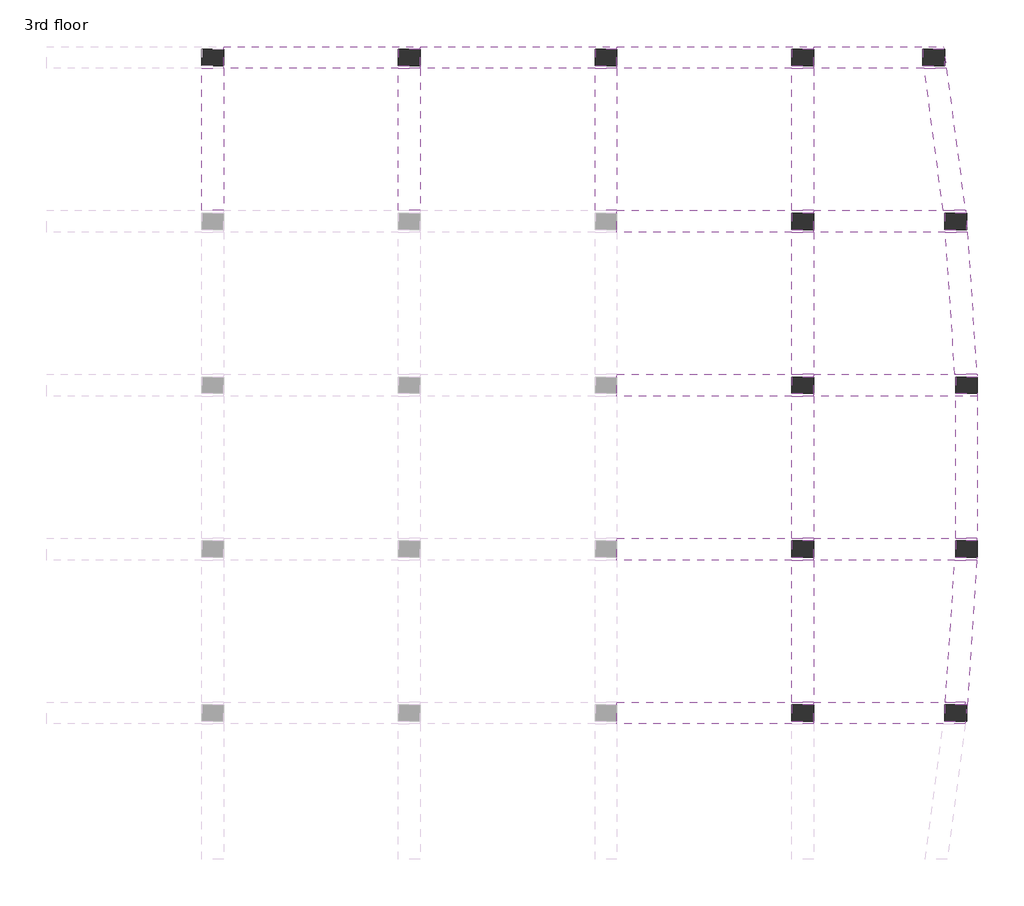
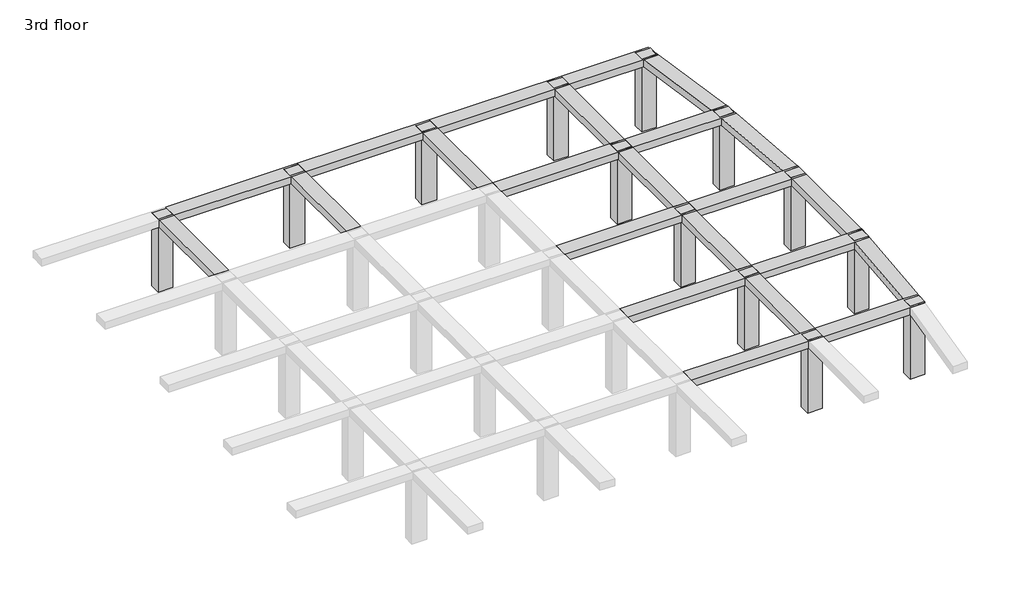
# One storey, part 3 of 3: 23 beams, 13 columns.
"""IFC4 building model written with IfcOpenShell, lengths in millimetres."""

from ifc_helpers import new_model, si_unit, frame, origin, place, context, project, spatial, polyline, outline, extrude, faceted_brep, element, save

model = new_model("IFC4")

# Units and contexts
model_context = context("Model", 3, world=origin())
ifc_project = project(units=[si_unit("LENGTHUNIT", "METRE", prefix="MILLI")], contexts=[model_context])

# Site, building, storey
site = spatial("IfcSite", under=ifc_project)
building = spatial("IfcBuilding", under=site)
storey = spatial("IfcBuildingStorey", under=building, Name="3rd floor", Elevation=9601.2)

# Beams
placement = place(None, origin())
element("IfcBeam", 1, ObjectType="Concrete-Rectangular Beam : 2' x2'", at=placement, inside=storey, context=model_context, shape_type="Brep", body=[
    faceted_brep([(-160.074232, 1680.7831222, 12801.6), (-160.074232, 1604.5831222, 12801.6), (-160.074232, 1147.3831222, 12801.6), (-160.074232, 1071.1831222, 12801.6), (4716.725768, 1071.1831222, 12801.6), (5326.325768, 1071.1831222, 12801.6), (5326.325768, 1147.3831222, 12801.6), (4716.725768, 1147.3831222, 12801.6), (4716.725768, 1604.5831222, 12801.6), (5326.325768, 1604.5831222, 12801.6), (5326.325768, 1680.7831222, 12801.6), (4716.725768, 1680.7831222, 12801.6), (-160.074232, 1071.1831222, 12496.8), (4716.725768, 1071.1831222, 12496.8), (5326.325768, 1071.1831222, 12496.8), (-160.074232, 1147.3831222, 12496.8), (-160.074232, 1604.5831222, 12496.8), (-160.074232, 1680.7831222, 12496.8), (4716.725768, 1680.7831222, 12496.8), (5326.325768, 1680.7831222, 12496.8), (5326.325768, 1604.5831222, 12496.8), (4716.725768, 1604.5831222, 12496.8), (4716.725768, 1147.3831222, 12496.8), (5326.325768, 1147.3831222, 12496.8)], [[[0, 1, 2, 3, 4, 5, 6, 7, 8, 9, 10, 11]], [[3, 12, 13, 14, 5, 4]], [[12, 15, 16, 17, 18, 19, 20, 21, 22, 23, 14, 13]], [[10, 19, 18, 17, 0, 11]], [[3, 2, 1, 0, 17, 16, 15, 12]], [[5, 14, 23, 6]], [[22, 7, 6, 23]], [[7, 22, 21, 8]], [[8, 21, 20, 9]], [[19, 10, 9, 20]]]),
])
element("IfcBeam", 2, ObjectType="Concrete-Rectangular Beam : 2' x2'", at=placement, inside=storey, context=model_context, shape_type="Brep", body=[
    faceted_brep([(9555.2251658, 1680.7831222, 12801.6), (9003.0522312, 1680.7831222, 12801.6), (5326.325768, 1680.7831222, 12801.6), (5326.325768, 1604.5831222, 12801.6), (5326.325768, 1147.3831222, 12801.6), (5326.325768, 1071.1831222, 12801.6), (8940.2370643, 1071.1831222, 12801.6), (9555.2251658, 1071.1831222, 12801.6), (9555.2251658, 1147.3831222, 12801.6), (8983.5457827, 1147.3831222, 12801.6), (8983.5457827, 1604.5831222, 12801.6), (9555.2251658, 1604.5831222, 12801.6), (9555.2251658, 1071.1831222, 12496.8), (5326.325768, 1071.1831222, 12496.8), (8940.2370643, 1071.1831222, 12496.8), (5326.325768, 1147.3831222, 12496.8), (5326.325768, 1604.5831222, 12496.8), (5326.325768, 1680.7831222, 12496.8), (9003.0522312, 1680.7831222, 12496.8), (9555.2251658, 1680.7831222, 12496.8), (9555.2251658, 1604.5831222, 12496.8), (8983.5457827, 1604.5831222, 12496.8), (8983.5457827, 1147.3831222, 12496.8), (9555.2251658, 1147.3831222, 12496.8)], [[[0, 1, 2, 3, 4, 5, 6, 7, 8, 9, 10, 11]], [[12, 7, 6, 5, 13, 14]], [[12, 14, 13, 15, 16, 17, 18, 19, 20, 21, 22, 23]], [[0, 19, 18, 17, 2, 1]], [[7, 12, 23, 8]], [[5, 4, 3, 2, 17, 16, 15, 13]], [[22, 9, 8, 23]], [[9, 22, 21, 10]], [[10, 21, 20, 11]], [[19, 0, 11, 20]]]),
])
element("IfcBeam", 3, ObjectType="Concrete-Rectangular Beam : 2' x2'", at=placement, inside=storey, context=model_context, shape_type="Brep", body=[
    faceted_brep([(-160.074232, 6252.7831222, 12801.6), (-160.074232, 6176.5831222, 12801.6), (-160.074232, 5719.3831222, 12801.6), (-160.074232, 5643.1831222, 12801.6), (4716.725768, 5643.1831222, 12801.6), (5326.325768, 5643.1831222, 12801.6), (5326.325768, 5719.3831222, 12801.6), (4716.725768, 5719.3831222, 12801.6), (4716.725768, 6176.5831222, 12801.6), (5326.325768, 6176.5831222, 12801.6), (5326.325768, 6252.7831222, 12801.6), (4716.725768, 6252.7831222, 12801.6), (-160.074232, 5643.1831222, 12496.8), (4716.725768, 5643.1831222, 12496.8), (5326.325768, 5643.1831222, 12496.8), (-160.074232, 5719.3831222, 12496.8), (-160.074232, 6176.5831222, 12496.8), (-160.074232, 6252.7831222, 12496.8), (4716.725768, 6252.7831222, 12496.8), (5326.325768, 6252.7831222, 12496.8), (5326.325768, 6176.5831222, 12496.8), (4716.725768, 6176.5831222, 12496.8), (4716.725768, 5719.3831222, 12496.8), (5326.325768, 5719.3831222, 12496.8)], [[[0, 1, 2, 3, 4, 5, 6, 7, 8, 9, 10, 11]], [[3, 12, 13, 14, 5, 4]], [[12, 15, 16, 17, 18, 19, 20, 21, 22, 23, 14, 13]], [[10, 19, 18, 17, 0, 11]], [[3, 2, 1, 0, 17, 16, 15, 12]], [[5, 14, 23, 6]], [[22, 7, 6, 23]], [[7, 22, 21, 8]], [[8, 21, 20, 9]], [[19, 10, 9, 20]]]),
])
element("IfcBeam", 4, ObjectType="Concrete-Rectangular Beam : 2' x2'", at=placement, inside=storey, context=model_context, shape_type="Brep", body=[
    faceted_brep([(9876.2389574, 6252.7831222, 12801.6), (9286.1454059, 6252.7831222, 12801.6), (5326.325768, 6252.7831222, 12801.6), (5326.325768, 6176.5831222, 12801.6), (5326.325768, 5719.3831222, 12801.6), (5326.325768, 5643.1831222, 12801.6), (9265.305238, 5643.1831222, 12801.6), (9876.2389574, 5643.1831222, 12801.6), (9876.2389574, 5719.3831222, 12801.6), (9286.1454059, 5719.3831222, 12801.6), (9286.1454059, 6176.5831222, 12801.6), (9876.2389574, 6176.5831222, 12801.6), (9876.2389574, 5643.1831222, 12496.8), (5326.325768, 5643.1831222, 12496.8), (9265.305238, 5643.1831222, 12496.8), (5326.325768, 5719.3831222, 12496.8), (5326.325768, 6176.5831222, 12496.8), (5326.325768, 6252.7831222, 12496.8), (9286.1454059, 6252.7831222, 12496.8), (9876.2389574, 6252.7831222, 12496.8), (9876.2389574, 6176.5831222, 12496.8), (9286.1454059, 6176.5831222, 12496.8), (9286.1454059, 5719.3831222, 12496.8), (9876.2389574, 5719.3831222, 12496.8)], [[[0, 1, 2, 3, 4, 5, 6, 7, 8, 9, 10, 11]], [[12, 7, 6, 5, 13, 14]], [[12, 14, 13, 15, 16, 17, 18, 19, 20, 21, 22, 23]], [[0, 19, 18, 17, 2, 1]], [[7, 12, 23, 8]], [[5, 4, 3, 2, 17, 16, 15, 13]], [[22, 9, 8, 23]], [[9, 22, 21, 10]], [[10, 21, 20, 11]], [[19, 0, 11, 20]]]),
])
element("IfcBeam", 5, ObjectType="Concrete-Rectangular Beam : 2' x2'", at=placement, inside=storey, context=model_context, shape_type="Brep", body=[
    faceted_brep([(-160.074232, 10824.7831222, 12801.6), (-160.074232, 10748.5831222, 12801.6), (-160.074232, 10291.3831222, 12801.6), (-160.074232, 10215.1831222, 12801.6), (4716.725768, 10215.1831222, 12801.6), (5326.325768, 10215.1831222, 12801.6), (5326.325768, 10291.3831222, 12801.6), (4716.725768, 10291.3831222, 12801.6), (4716.725768, 10748.5831222, 12801.6), (5326.325768, 10748.5831222, 12801.6), (5326.325768, 10824.7831222, 12801.6), (4716.725768, 10824.7831222, 12801.6), (-160.074232, 10215.1831222, 12496.8), (4716.725768, 10215.1831222, 12496.8), (5326.325768, 10215.1831222, 12496.8), (-160.074232, 10291.3831222, 12496.8), (-160.074232, 10748.5831222, 12496.8), (-160.074232, 10824.7831222, 12496.8), (4716.725768, 10824.7831222, 12496.8), (5326.325768, 10824.7831222, 12496.8), (5326.325768, 10748.5831222, 12496.8), (4716.725768, 10748.5831222, 12496.8), (4716.725768, 10291.3831222, 12496.8), (5326.325768, 10291.3831222, 12496.8)], [[[0, 1, 2, 3, 4, 5, 6, 7, 8, 9, 10, 11]], [[3, 12, 13, 14, 5, 4]], [[12, 15, 16, 17, 18, 19, 20, 21, 22, 23, 14, 13]], [[10, 19, 18, 17, 0, 11]], [[3, 2, 1, 0, 17, 16, 15, 12]], [[5, 14, 23, 6]], [[22, 7, 6, 23]], [[7, 22, 21, 8]], [[8, 21, 20, 9]], [[19, 10, 9, 20]]]),
])
element("IfcBeam", 6, ObjectType="Concrete-Rectangular Beam : 2' x2'", at=placement, inside=storey, context=model_context, shape_type="Brep", body=[
    faceted_brep([(9895.7454059, 10824.7831222, 12801.6), (9876.2389574, 10824.7831222, 12801.6), (9265.305238, 10824.7831222, 12801.6), (5326.325768, 10824.7831222, 12801.6), (5326.325768, 10748.5831222, 12801.6), (5326.325768, 10291.3831222, 12801.6), (5326.325768, 10215.1831222, 12801.6), (9895.7454059, 10215.1831222, 12801.6), (9895.7454059, 10291.3831222, 12801.6), (9286.1454059, 10291.3831222, 12801.6), (9286.1454059, 10748.5831222, 12801.6), (9895.7454059, 10748.5831222, 12801.6), (9895.7454059, 10215.1831222, 12496.8), (5326.325768, 10215.1831222, 12496.8), (5326.325768, 10291.3831222, 12496.8), (5326.325768, 10748.5831222, 12496.8), (5326.325768, 10824.7831222, 12496.8), (9265.305238, 10824.7831222, 12496.8), (9876.2389574, 10824.7831222, 12496.8), (9895.7454059, 10824.7831222, 12496.8), (9895.7454059, 10748.5831222, 12496.8), (9286.1454059, 10748.5831222, 12496.8), (9286.1454059, 10291.3831222, 12496.8), (9895.7454059, 10291.3831222, 12496.8)], [[[0, 1, 2, 3, 4, 5, 6, 7, 8, 9, 10, 11]], [[12, 7, 6, 13]], [[12, 13, 14, 15, 16, 17, 18, 19, 20, 21, 22, 23]], [[0, 19, 18, 17, 16, 3, 2, 1]], [[7, 12, 23, 8]], [[6, 5, 4, 3, 16, 15, 14, 13]], [[22, 9, 8, 23]], [[9, 22, 21, 10]], [[10, 21, 20, 11]], [[19, 0, 11, 20]]]),
])
element("IfcBeam", 7, ObjectType="Concrete-Rectangular Beam : 2' x2'", at=placement, inside=storey, context=model_context, shape_type="Brep", body=[
    faceted_brep([(-160.074232, 15396.7831222, 12801.6), (-160.074232, 15320.5831222, 12801.6), (-160.074232, 14863.3831222, 12801.6), (-160.074232, 14787.1831222, 12801.6), (4716.725768, 14787.1831222, 12801.6), (5326.325768, 14787.1831222, 12801.6), (5326.325768, 14863.3831222, 12801.6), (4716.725768, 14863.3831222, 12801.6), (4716.725768, 15320.5831222, 12801.6), (5326.325768, 15320.5831222, 12801.6), (5326.325768, 15396.7831222, 12801.6), (4716.725768, 15396.7831222, 12801.6), (-160.074232, 14787.1831222, 12496.8), (4716.725768, 14787.1831222, 12496.8), (5326.325768, 14787.1831222, 12496.8), (-160.074232, 14863.3831222, 12496.8), (-160.074232, 15320.5831222, 12496.8), (-160.074232, 15396.7831222, 12496.8), (4716.725768, 15396.7831222, 12496.8), (5326.325768, 15396.7831222, 12496.8), (5326.325768, 15320.5831222, 12496.8), (4716.725768, 15320.5831222, 12496.8), (4716.725768, 14863.3831222, 12496.8), (5326.325768, 14863.3831222, 12496.8)], [[[0, 1, 2, 3, 4, 5, 6, 7, 8, 9, 10, 11]], [[3, 12, 13, 14, 5, 4]], [[12, 15, 16, 17, 18, 19, 20, 21, 22, 23, 14, 13]], [[10, 19, 18, 17, 0, 11]], [[3, 2, 1, 0, 17, 16, 15, 12]], [[5, 14, 23, 6]], [[22, 7, 6, 23]], [[7, 22, 21, 8]], [[8, 21, 20, 9]], [[19, 10, 9, 20]]]),
])
element("IfcBeam", 8, ObjectType="Concrete-Rectangular Beam : 2' x2'", at=placement, inside=storey, context=model_context, shape_type="Brep", body=[
    faceted_brep([(9573.6393342, 15396.7831222, 12801.6), (9555.2251658, 15396.7831222, 12801.6), (8940.2370643, 15396.7831222, 12801.6), (5326.325768, 15396.7831222, 12801.6), (5326.325768, 15320.5831222, 12801.6), (5326.325768, 14863.3831222, 12801.6), (5326.325768, 14787.1831222, 12801.6), (9003.0522312, 14787.1831222, 12801.6), (9613.9859506, 14787.1831222, 12801.6), (9593.1457827, 15102.0587543, 12801.6), (9593.1457827, 14863.3831222, 12801.6), (8983.5457827, 14863.3831222, 12801.6), (8983.5457827, 15320.5831222, 12801.6), (9578.6826612, 15320.5831222, 12801.6), (9613.9859506, 14787.1831222, 12496.8), (5326.325768, 14787.1831222, 12496.8), (9003.0522312, 14787.1831222, 12496.8), (5326.325768, 14863.3831222, 12496.8), (5326.325768, 15320.5831222, 12496.8), (5326.325768, 15396.7831222, 12496.8), (8940.2370643, 15396.7831222, 12496.8), (9555.2251658, 15396.7831222, 12496.8), (9573.6393342, 15396.7831222, 12496.8), (9578.6826612, 15320.5831222, 12496.8), (8983.5457827, 15320.5831222, 12496.8), (8983.5457827, 14863.3831222, 12496.8), (9593.1457827, 14863.3831222, 12496.8), (9593.1457827, 15102.0587543, 12496.8)], [[[0, 1, 2, 3, 4, 5, 6, 7, 8, 9, 10, 11, 12, 13]], [[14, 8, 7, 6, 15, 16]], [[14, 16, 15, 17, 18, 19, 20, 21, 22, 23, 24, 25, 26, 27]], [[0, 22, 21, 20, 19, 3, 2, 1]], [[8, 14, 27, 9]], [[6, 5, 4, 3, 19, 18, 17, 15]], [[26, 10, 9, 27]], [[10, 26, 25, 11]], [[11, 25, 24, 12]], [[12, 24, 23, 13]], [[22, 0, 13, 23]]]),
])
element("IfcBeam", 9, ObjectType="Concrete-Rectangular Beam : 2' x2'", at=placement, inside=storey, context=model_context, shape_type="Brep", body=[
    faceted_brep([(-11132.874232, 19968.7831222, 12801.6), (-11132.874232, 19892.5831222, 12801.6), (-11132.874232, 19435.3831222, 12801.6), (-11132.874232, 19359.1831222, 12801.6), (-6256.074232, 19359.1831222, 12801.6), (-5646.474232, 19359.1831222, 12801.6), (-5646.474232, 19435.3831222, 12801.6), (-6256.074232, 19435.3831222, 12801.6), (-6256.074232, 19892.5831222, 12801.6), (-5646.474232, 19892.5831222, 12801.6), (-5646.474232, 19968.7831222, 12801.6), (-11132.874232, 19359.1831222, 12496.8), (-6256.074232, 19359.1831222, 12496.8), (-5646.474232, 19359.1831222, 12496.8), (-11132.874232, 19435.3831222, 12496.8), (-11132.874232, 19892.5831222, 12496.8), (-11132.874232, 19968.7831222, 12496.8), (-5646.474232, 19968.7831222, 12496.8), (-5646.474232, 19892.5831222, 12496.8), (-6256.074232, 19892.5831222, 12496.8), (-6256.074232, 19435.3831222, 12496.8), (-5646.474232, 19435.3831222, 12496.8)], [[[0, 1, 2, 3, 4, 5, 6, 7, 8, 9, 10]], [[3, 11, 12, 13, 5, 4]], [[11, 14, 15, 16, 17, 18, 19, 20, 21, 13, 12]], [[10, 17, 16, 0]], [[3, 2, 1, 0, 16, 15, 14, 11]], [[5, 13, 21, 6]], [[20, 7, 6, 21]], [[7, 20, 19, 8]], [[8, 19, 18, 9]], [[17, 10, 9, 18]]]),
])
element("IfcBeam", 10, ObjectType="Concrete-Rectangular Beam : 2' x2'", at=placement, inside=storey, context=model_context, shape_type="Brep", body=[
    faceted_brep([(-160.074232, 19968.7831222, 12801.6), (-5646.474232, 19968.7831222, 12801.6), (-5646.474232, 19892.5831222, 12801.6), (-5646.474232, 19435.3831222, 12801.6), (-5646.474232, 19359.1831222, 12801.6), (-769.674232, 19359.1831222, 12801.6), (-160.074232, 19359.1831222, 12801.6), (-160.074232, 19435.3831222, 12801.6), (-769.674232, 19435.3831222, 12801.6), (-769.674232, 19892.5831222, 12801.6), (-160.074232, 19892.5831222, 12801.6), (-160.074232, 19359.1831222, 12496.8), (-5646.474232, 19359.1831222, 12496.8), (-769.674232, 19359.1831222, 12496.8), (-5646.474232, 19435.3831222, 12496.8), (-5646.474232, 19892.5831222, 12496.8), (-5646.474232, 19968.7831222, 12496.8), (-160.074232, 19968.7831222, 12496.8), (-160.074232, 19892.5831222, 12496.8), (-769.674232, 19892.5831222, 12496.8), (-769.674232, 19435.3831222, 12496.8), (-160.074232, 19435.3831222, 12496.8)], [[[0, 1, 2, 3, 4, 5, 6, 7, 8, 9, 10]], [[11, 6, 5, 4, 12, 13]], [[11, 13, 12, 14, 15, 16, 17, 18, 19, 20, 21]], [[0, 17, 16, 1]], [[6, 11, 21, 7]], [[4, 3, 2, 1, 16, 15, 14, 12]], [[20, 8, 7, 21]], [[8, 20, 19, 9]], [[9, 19, 18, 10]], [[17, 0, 10, 18]]]),
])
element("IfcBeam", 11, ObjectType="Concrete-Rectangular Beam : 2' x2'", at=placement, inside=storey, context=model_context, shape_type="Brep", body=[
    faceted_brep([(-160.074232, 19968.7831222, 12801.6), (-160.074232, 19892.5831222, 12801.6), (-160.074232, 19435.3831222, 12801.6), (-160.074232, 19359.1831222, 12801.6), (4716.725768, 19359.1831222, 12801.6), (5326.325768, 19359.1831222, 12801.6), (5326.325768, 19435.3831222, 12801.6), (4716.725768, 19435.3831222, 12801.6), (4716.725768, 19892.5831222, 12801.6), (5326.325768, 19892.5831222, 12801.6), (5326.325768, 19968.7831222, 12801.6), (-160.074232, 19359.1831222, 12496.8), (4716.725768, 19359.1831222, 12496.8), (5326.325768, 19359.1831222, 12496.8), (-160.074232, 19435.3831222, 12496.8), (-160.074232, 19892.5831222, 12496.8), (-160.074232, 19968.7831222, 12496.8), (5326.325768, 19968.7831222, 12496.8), (5326.325768, 19892.5831222, 12496.8), (4716.725768, 19892.5831222, 12496.8), (4716.725768, 19435.3831222, 12496.8), (5326.325768, 19435.3831222, 12496.8)], [[[0, 1, 2, 3, 4, 5, 6, 7, 8, 9, 10]], [[3, 11, 12, 13, 5, 4]], [[11, 14, 15, 16, 17, 18, 19, 20, 21, 13, 12]], [[10, 17, 16, 0]], [[3, 2, 1, 0, 16, 15, 14, 11]], [[5, 13, 21, 6]], [[20, 7, 6, 21]], [[7, 20, 19, 8]], [[8, 19, 18, 9]], [[17, 10, 9, 18]]]),
])
element("IfcBeam", 12, ObjectType="Concrete-Rectangular Beam : 2' x2'", at=placement, inside=storey, context=model_context, shape_type="Brep", body=[
    faceted_brep([(5326.325768, 19968.7831222, 12801.6), (5326.325768, 19892.5831222, 12801.6), (5326.325768, 19435.3831222, 12801.6), (5326.325768, 19359.1831222, 12801.6), (8412.2463849, 19359.1831222, 12801.6), (9027.2344863, 19359.1831222, 12801.6), (8983.925768, 19684.2011052, 12801.6), (8983.925768, 19435.3831222, 12801.6), (8374.325768, 19435.3831222, 12801.6), (8374.325768, 19892.5831222, 12801.6), (8956.158818, 19892.5831222, 12801.6), (8946.005151, 19968.7831222, 12801.6), (5326.325768, 19359.1831222, 12496.8), (8412.2463849, 19359.1831222, 12496.8), (9027.2344863, 19359.1831222, 12496.8), (5326.325768, 19435.3831222, 12496.8), (5326.325768, 19892.5831222, 12496.8), (5326.325768, 19968.7831222, 12496.8), (8946.005151, 19968.7831222, 12496.8), (8956.158818, 19892.5831222, 12496.8), (8374.325768, 19892.5831222, 12496.8), (8374.325768, 19435.3831222, 12496.8), (8983.925768, 19435.3831222, 12496.8), (8983.925768, 19684.2011052, 12496.8)], [[[0, 1, 2, 3, 4, 5, 6, 7, 8, 9, 10, 11]], [[3, 12, 13, 14, 5, 4]], [[12, 15, 16, 17, 18, 19, 20, 21, 22, 23, 14, 13]], [[11, 18, 17, 0]], [[3, 2, 1, 0, 17, 16, 15, 12]], [[5, 14, 23, 6]], [[22, 7, 6, 23]], [[7, 22, 21, 8]], [[8, 21, 20, 9]], [[9, 20, 19, 10]], [[18, 11, 10, 19]]]),
])
element("IfcBeam", 13, ObjectType="Concrete-Rectangular Beam : 2' x2'", at=placement, inside=storey, context=model_context, shape_type="SweptSolid", body=[
    extrude(outline(polyline([(-11132.874232, 15396.7831222), (-11742.474232, 15396.7831222), (-11742.474232, 19359.1831222), (-11132.874232, 19359.1831222), (-11132.874232, 15396.7831222)])), frame((0.0, 0.0, 12496.8), z_axis=(0.0, 0.0, 1.0), x_axis=(1.0, 0.0, 0.0)), (0.0, 0.0, 1.0), 304.8),
])
element("IfcBeam", 14, ObjectType="Concrete-Rectangular Beam : 2' x2'", at=placement, inside=storey, context=model_context, shape_type="SweptSolid", body=[
    extrude(outline(polyline([(-5646.474232, 15396.7831222), (-6256.074232, 15396.7831222), (-6256.074232, 19359.1831222), (-5646.474232, 19359.1831222), (-5646.474232, 15396.7831222)])), frame((0.0, 0.0, 12496.8), z_axis=(0.0, 0.0, 1.0), x_axis=(1.0, 0.0, 0.0)), (0.0, 0.0, 1.0), 304.8),
])
element("IfcBeam", 15, ObjectType="Concrete-Rectangular Beam : 2' x2'", at=placement, inside=storey, context=model_context, shape_type="SweptSolid", body=[
    extrude(outline(polyline([(-160.074232, 15396.7831222), (-769.674232, 15396.7831222), (-769.674232, 19359.1831222), (-160.074232, 19359.1831222), (-160.074232, 15396.7831222)])), frame((0.0, 0.0, 12496.8), z_axis=(0.0, 0.0, 1.0), x_axis=(1.0, 0.0, 0.0)), (0.0, 0.0, 1.0), 304.8),
])
element("IfcBeam", 16, ObjectType="Concrete-Rectangular Beam : 2' x2'", at=placement, inside=storey, context=model_context, shape_type="SweptSolid", body=[
    extrude(outline(polyline([(5326.325768, 1680.7831222), (4716.725768, 1680.7831222), (4716.725768, 5643.1831222), (5326.325768, 5643.1831222), (5326.325768, 1680.7831222)])), frame((0.0, 0.0, 12496.8), z_axis=(0.0, 0.0, 1.0), x_axis=(1.0, 0.0, 0.0)), (0.0, 0.0, 1.0), 304.8),
])
element("IfcBeam", 17, ObjectType="Concrete-Rectangular Beam : 2' x2'", at=placement, inside=storey, context=model_context, shape_type="SweptSolid", body=[
    extrude(outline(polyline([(4716.725768, 10215.1831222), (5326.325768, 10215.1831222), (5326.325768, 6252.7831222), (4716.725768, 6252.7831222), (4716.725768, 10215.1831222)])), frame((0.0, 0.0, 12496.8), z_axis=(0.0, 0.0, 1.0), x_axis=(1.0, 0.0, 0.0)), (0.0, 0.0, 1.0), 304.8),
])
element("IfcBeam", 18, ObjectType="Concrete-Rectangular Beam : 2' x2'", at=placement, inside=storey, context=model_context, shape_type="SweptSolid", body=[
    extrude(outline(polyline([(4716.725768, 14787.1831222), (5326.325768, 14787.1831222), (5326.325768, 10824.7831222), (4716.725768, 10824.7831222), (4716.725768, 14787.1831222)])), frame((0.0, 0.0, 12496.8), z_axis=(0.0, 0.0, 1.0), x_axis=(1.0, 0.0, 0.0)), (0.0, 0.0, 1.0), 304.8),
])
element("IfcBeam", 19, ObjectType="Concrete-Rectangular Beam : 2' x2'", at=placement, inside=storey, context=model_context, shape_type="SweptSolid", body=[
    extrude(outline(polyline([(5326.325768, 15396.7831222), (4716.725768, 15396.7831222), (4716.725768, 19359.1831222), (5326.325768, 19359.1831222), (5326.325768, 15396.7831222)])), frame((0.0, 0.0, 12496.8), z_axis=(0.0, 0.0, 1.0), x_axis=(1.0, 0.0, 0.0)), (0.0, 0.0, 1.0), 304.8),
])
element("IfcBeam", 20, ObjectType="Concrete-Rectangular Beam : 2' x2'", at=placement, inside=storey, context=model_context, shape_type="Brep", body=[
    faceted_brep([(9916.5855738, 6252.7831222, 12801.6), (9895.7454059, 6252.7831222, 12801.6), (9876.2389574, 6252.7831222, 12801.6), (9876.2389574, 6176.5831222, 12801.6), (9895.7454059, 6176.5831222, 12801.6), (9895.7454059, 5937.9074901, 12801.6), (9916.5855738, 6252.7831222, 12496.8), (9895.7454059, 5937.9074901, 12496.8), (9876.2389574, 6252.7831222, 12496.8), (9895.7454059, 6252.7831222, 12496.8), (9895.7454059, 6176.5831222, 12496.8), (9876.2389574, 6176.5831222, 12496.8)], [[[0, 1, 2, 3, 4, 5]], [[6, 0, 5, 7]], [[8, 9, 6, 7, 10, 11]], [[0, 6, 9, 8, 2, 1]], [[4, 10, 7, 5]], [[10, 4, 3, 11]], [[2, 8, 11, 3]]]),
    faceted_brep([(9003.0522312, 1680.7831222, 12496.8), (9003.0522312, 1680.7831222, 12801.6), (9265.305238, 5643.1831222, 12801.6), (9265.305238, 5643.1831222, 12496.8), (9021.4663996, 1680.7831222, 12496.8), (9555.2251658, 1680.7831222, 12496.8), (9555.2251658, 1680.7831222, 12801.6), (9021.4663996, 1680.7831222, 12801.6), (9876.2389574, 5643.1831222, 12801.6), (9876.2389574, 5643.1831222, 12496.8), (9876.2389574, 5719.3831222, 12801.6), (9876.2389574, 5719.3831222, 12496.8), (9555.2251658, 1604.5831222, 12801.6), (9593.1457827, 1604.5831222, 12801.6), (9593.1457827, 1365.9074901, 12801.6), (9593.1457827, 1365.9074901, 12496.8), (9593.1457827, 1604.5831222, 12496.8), (9555.2251658, 1604.5831222, 12496.8), (9881.2822845, 5719.3831222, 12801.6), (9881.2822845, 5719.3831222, 12496.8)], [[[0, 1, 2, 3]], [[1, 0, 4, 5, 6, 7]], [[2, 8, 9, 3]], [[9, 8, 10, 11]], [[8, 2, 1, 7, 6, 12, 13, 14]], [[3, 9, 15, 16, 17, 5, 4, 0]], [[13, 16, 15, 14]], [[16, 13, 12, 17]], [[6, 5, 17, 12]], [[10, 18, 19, 11]], [[10, 8, 18]], [[8, 14, 15, 9, 19, 18]], [[19, 9, 11]]]),
    faceted_brep([(9555.2251658, 1071.1831222, 12801.6), (9555.2251658, 1071.1831222, 12496.8), (9565.3788327, 1147.3831222, 12496.8), (9565.3788327, 1147.3831222, 12801.6), (9555.2251658, 1147.3831222, 12801.6), (9555.2251658, 1147.3831222, 12496.8)], [[[0, 1, 2, 3]], [[1, 0, 4, 5]], [[3, 2, 5, 4]], [[4, 0, 3]], [[2, 1, 5]]]),
])
element("IfcBeam", 21, ObjectType="Concrete-Rectangular Beam : 2' x2'", at=placement, inside=storey, context=model_context, shape_type="Brep", body=[
    faceted_brep([(9895.7454059, 10824.7831222, 12801.6), (9876.2389574, 10824.7831222, 12801.6), (9286.1454059, 10824.7831222, 12801.6), (9286.1454059, 10748.5831222, 12801.6), (9895.7454059, 10748.5831222, 12801.6), (9895.7454059, 10824.7831222, 12496.8), (9895.7454059, 10748.5831222, 12496.8), (9286.1454059, 10824.7831222, 12496.8), (9876.2389574, 10824.7831222, 12496.8), (9286.1454059, 10748.5831222, 12496.8)], [[[0, 1, 2, 3, 4]], [[5, 0, 4, 6]], [[7, 8, 5, 6, 9]], [[2, 7, 9, 3]], [[2, 1, 0, 5, 8, 7]], [[4, 3, 9, 6]]]),
    faceted_brep([(9286.1454059, 6252.7831222, 12801.6), (9286.1454059, 6252.7831222, 12496.8), (9876.2389574, 6252.7831222, 12496.8), (9895.7454059, 6252.7831222, 12496.8), (9895.7454059, 6252.7831222, 12801.6), (9876.2389574, 6252.7831222, 12801.6), (9286.1454059, 10291.3831222, 12801.6), (9895.7454059, 10291.3831222, 12801.6), (9895.7454059, 10291.3831222, 12496.8), (9286.1454059, 10291.3831222, 12496.8)], [[[0, 1, 2, 3, 4, 5]], [[6, 7, 8, 9]], [[0, 5, 4, 7, 6]], [[4, 3, 8, 7]], [[3, 2, 1, 9, 8]], [[1, 0, 6, 9]]]),
])
element("IfcBeam", 22, ObjectType="Concrete-Rectangular Beam : 2' x2'", at=placement, inside=storey, context=model_context, shape_type="Brep", body=[
    faceted_brep([(9613.9859506, 14787.1831222, 12801.6), (9003.0522312, 14787.1831222, 12801.6), (9265.305238, 10824.7831222, 12801.6), (9286.1454059, 10824.7831222, 12801.6), (9876.2389574, 10824.7831222, 12801.6), (9613.9859506, 14787.1831222, 12496.8), (9876.2389574, 10824.7831222, 12496.8), (9003.0522312, 14787.1831222, 12496.8), (9286.1454059, 10824.7831222, 12496.8), (9265.305238, 10824.7831222, 12496.8)], [[[0, 1, 2, 3, 4]], [[5, 0, 4, 6]], [[7, 5, 6, 8, 9]], [[1, 7, 9, 2]], [[1, 0, 5, 7]], [[4, 3, 2, 9, 8, 6]]]),
])
element("IfcBeam", 23, ObjectType="Concrete-Rectangular Beam : 2' x2'", at=placement, inside=storey, context=model_context, shape_type="SweptSolid", body=[
    extrude(outline(polyline([(8412.2463849, 19359.1831222), (9027.2344863, 19359.1831222), (9555.2251658, 15396.7831222), (8940.2370643, 15396.7831222), (8412.2463849, 19359.1831222)])), frame((0.0, 0.0, 12496.8), z_axis=(0.0, 0.0, 1.0), x_axis=(1.0, 0.0, 0.0)), (0.0, 0.0, 1.0), 304.8),
])

# Columns
element("IfcColumn", 24, ObjectType="Concrete-Rectangular-Column : 12 x 18", at=placement, inside=storey, context=model_context, shape_type="SweptSolid", body=[
    extrude(outline(polyline([(5326.325768, 1604.5831222), (5326.325768, 1147.3831222), (4716.725768, 1147.3831222), (4716.725768, 1604.5831222), (5326.325768, 1604.5831222)])), frame((0.0, 0.0, 9601.2), z_axis=(0.0, 0.0, 1.0), x_axis=(1.0, 0.0, 0.0)), (0.0, 0.0, 1.0), 3200.4),
])
element("IfcColumn", 25, ObjectType="Concrete-Rectangular-Column : 12 x 18", at=placement, inside=storey, context=model_context, shape_type="SweptSolid", body=[
    extrude(outline(polyline([(9593.1457827, 1604.5831222), (9593.1457827, 1147.3831222), (8983.5457827, 1147.3831222), (8983.5457827, 1604.5831222), (9593.1457827, 1604.5831222)])), frame((0.0, 0.0, 9601.2), z_axis=(0.0, 0.0, 1.0), x_axis=(1.0, 0.0, 0.0)), (0.0, 0.0, 1.0), 3200.4),
])
element("IfcColumn", 26, ObjectType="Concrete-Rectangular-Column : 12 x 18", at=placement, inside=storey, context=model_context, shape_type="SweptSolid", body=[
    extrude(outline(polyline([(5326.325768, 6176.5831222), (5326.325768, 5719.3831222), (4716.725768, 5719.3831222), (4716.725768, 6176.5831222), (5326.325768, 6176.5831222)])), frame((0.0, 0.0, 9601.2), z_axis=(0.0, 0.0, 1.0), x_axis=(1.0, 0.0, 0.0)), (0.0, 0.0, 1.0), 3200.4),
])
element("IfcColumn", 27, ObjectType="Concrete-Rectangular-Column : 12 x 18", at=placement, inside=storey, context=model_context, shape_type="SweptSolid", body=[
    extrude(outline(polyline([(9895.7454059, 6176.5831222), (9895.7454059, 5719.3831222), (9286.1454059, 5719.3831222), (9286.1454059, 6176.5831222), (9895.7454059, 6176.5831222)])), frame((0.0, 0.0, 9601.2), z_axis=(0.0, 0.0, 1.0), x_axis=(1.0, 0.0, 0.0)), (0.0, 0.0, 1.0), 3200.4),
])
element("IfcColumn", 28, ObjectType="Concrete-Rectangular-Column : 12 x 18", at=placement, inside=storey, context=model_context, shape_type="SweptSolid", body=[
    extrude(outline(polyline([(5326.325768, 10748.5831222), (5326.325768, 10291.3831222), (4716.725768, 10291.3831222), (4716.725768, 10748.5831222), (5326.325768, 10748.5831222)])), frame((0.0, 0.0, 9601.2), z_axis=(0.0, 0.0, 1.0), x_axis=(1.0, 0.0, 0.0)), (0.0, 0.0, 1.0), 3200.4),
])
element("IfcColumn", 29, ObjectType="Concrete-Rectangular-Column : 12 x 18", at=placement, inside=storey, context=model_context, shape_type="SweptSolid", body=[
    extrude(outline(polyline([(9895.7454059, 10748.5831222), (9895.7454059, 10291.3831222), (9286.1454059, 10291.3831222), (9286.1454059, 10748.5831222), (9895.7454059, 10748.5831222)])), frame((0.0, 0.0, 9601.2), z_axis=(0.0, 0.0, 1.0), x_axis=(1.0, 0.0, 0.0)), (0.0, 0.0, 1.0), 3200.4),
])
element("IfcColumn", 30, ObjectType="Concrete-Rectangular-Column : 12 x 18", at=placement, inside=storey, context=model_context, shape_type="SweptSolid", body=[
    extrude(outline(polyline([(5326.325768, 15320.5831222), (5326.325768, 14863.3831222), (4716.725768, 14863.3831222), (4716.725768, 15320.5831222), (5326.325768, 15320.5831222)])), frame((0.0, 0.0, 9601.2), z_axis=(0.0, 0.0, 1.0), x_axis=(1.0, 0.0, 0.0)), (0.0, 0.0, 1.0), 3200.4),
])
element("IfcColumn", 31, ObjectType="Concrete-Rectangular-Column : 12 x 18", at=placement, inside=storey, context=model_context, shape_type="SweptSolid", body=[
    extrude(outline(polyline([(9593.1457827, 15320.5831222), (9593.1457827, 14863.3831222), (8983.5457827, 14863.3831222), (8983.5457827, 15320.5831222), (9593.1457827, 15320.5831222)])), frame((0.0, 0.0, 9601.2), z_axis=(0.0, 0.0, 1.0), x_axis=(1.0, 0.0, 0.0)), (0.0, 0.0, 1.0), 3200.4),
])
element("IfcColumn", 32, ObjectType="Concrete-Rectangular-Column : 12 x 18", at=placement, inside=storey, context=model_context, shape_type="SweptSolid", body=[
    extrude(outline(polyline([(-11132.874232, 19892.5831222), (-11132.874232, 19435.3831222), (-11742.474232, 19435.3831222), (-11742.474232, 19892.5831222), (-11132.874232, 19892.5831222)])), frame((0.0, 0.0, 9601.2), z_axis=(0.0, 0.0, 1.0), x_axis=(1.0, 0.0, 0.0)), (0.0, 0.0, 1.0), 3200.4),
])
element("IfcColumn", 33, ObjectType="Concrete-Rectangular-Column : 12 x 18", at=placement, inside=storey, context=model_context, shape_type="SweptSolid", body=[
    extrude(outline(polyline([(-5646.474232, 19892.5831222), (-5646.474232, 19435.3831222), (-6256.074232, 19435.3831222), (-6256.074232, 19892.5831222), (-5646.474232, 19892.5831222)])), frame((0.0, 0.0, 9601.2), z_axis=(0.0, 0.0, 1.0), x_axis=(1.0, 0.0, 0.0)), (0.0, 0.0, 1.0), 3200.4),
])
element("IfcColumn", 34, ObjectType="Concrete-Rectangular-Column : 12 x 18", at=placement, inside=storey, context=model_context, shape_type="SweptSolid", body=[
    extrude(outline(polyline([(-160.074232, 19892.5831222), (-160.074232, 19435.3831222), (-769.674232, 19435.3831222), (-769.674232, 19892.5831222), (-160.074232, 19892.5831222)])), frame((0.0, 0.0, 9601.2), z_axis=(0.0, 0.0, 1.0), x_axis=(1.0, 0.0, 0.0)), (0.0, 0.0, 1.0), 3200.4),
])
element("IfcColumn", 35, ObjectType="Concrete-Rectangular-Column : 12 x 18", at=placement, inside=storey, context=model_context, shape_type="SweptSolid", body=[
    extrude(outline(polyline([(5326.325768, 19892.5831222), (5326.325768, 19435.3831222), (4716.725768, 19435.3831222), (4716.725768, 19892.5831222), (5326.325768, 19892.5831222)])), frame((0.0, 0.0, 9601.2), z_axis=(0.0, 0.0, 1.0), x_axis=(1.0, 0.0, 0.0)), (0.0, 0.0, 1.0), 3200.4),
])
element("IfcColumn", 36, ObjectType="Concrete-Rectangular-Column : 12 x 18", at=placement, inside=storey, context=model_context, shape_type="SweptSolid", body=[
    extrude(outline(polyline([(8983.925768, 19892.5831222), (8983.925768, 19435.3831222), (8374.325768, 19435.3831222), (8374.325768, 19892.5831222), (8983.925768, 19892.5831222)])), frame((0.0, 0.0, 9601.2), z_axis=(0.0, 0.0, 1.0), x_axis=(1.0, 0.0, 0.0)), (0.0, 0.0, 1.0), 3200.4),
])

save(model, "model.ifc")

# Revit data of these elements
# Type "Concrete-Rectangular Beam : 2' x2'"
#   Assembly Code = "B10"
#   Length [instance default] = 5' - 0"
#   b = 2' - 0"
#   h = 1' - 0"
#   Structural Material [instance default] = Concrete, Cast-in-Place gray
# Type "Concrete-Rectangular-Column : 12 x 18"
#   Assembly Code = "B10"
#   b = 2' - 0"
#   h = 1' - 6"
#   Structural Material [instance default] = Concrete, Cast-in-Place gray
# Elements 1, 2, 3, 4, 5, 6, 7, 8, 9, 10, 11, 12, 13, 14, 15, 16, 17, 18, 19, 20, 21, 22, 23 (IfcBeam, "Concrete-Rectangular Beam : 2' x2'")
#   Structural Material = Concrete, Precast (2)
#   Phase Created = New Construction
#   Materials on its faces: "Concrete, Precast (2)"
# Elements 24, 25, 26, 27, 28, 29, 30, 31, 32, 33, 34, 35, 36 (IfcColumn, "Concrete-Rectangular-Column : 12 x 18")
#   Phase Created = New Construction
#   Materials on its faces: "Concrete, Cast-in-Place gray"
# Materials
#   "Concrete, Cast-in-Place gray": class "Concrete", colour RGB 192 192 192, transparency 0, Description = "Cast-in-place concrete", Cost = 0
#   "Concrete, Precast (2)": class "Concrete", colour RGB 198 187 187, transparency 0, Description = "Precast concrete", Cost = 0
